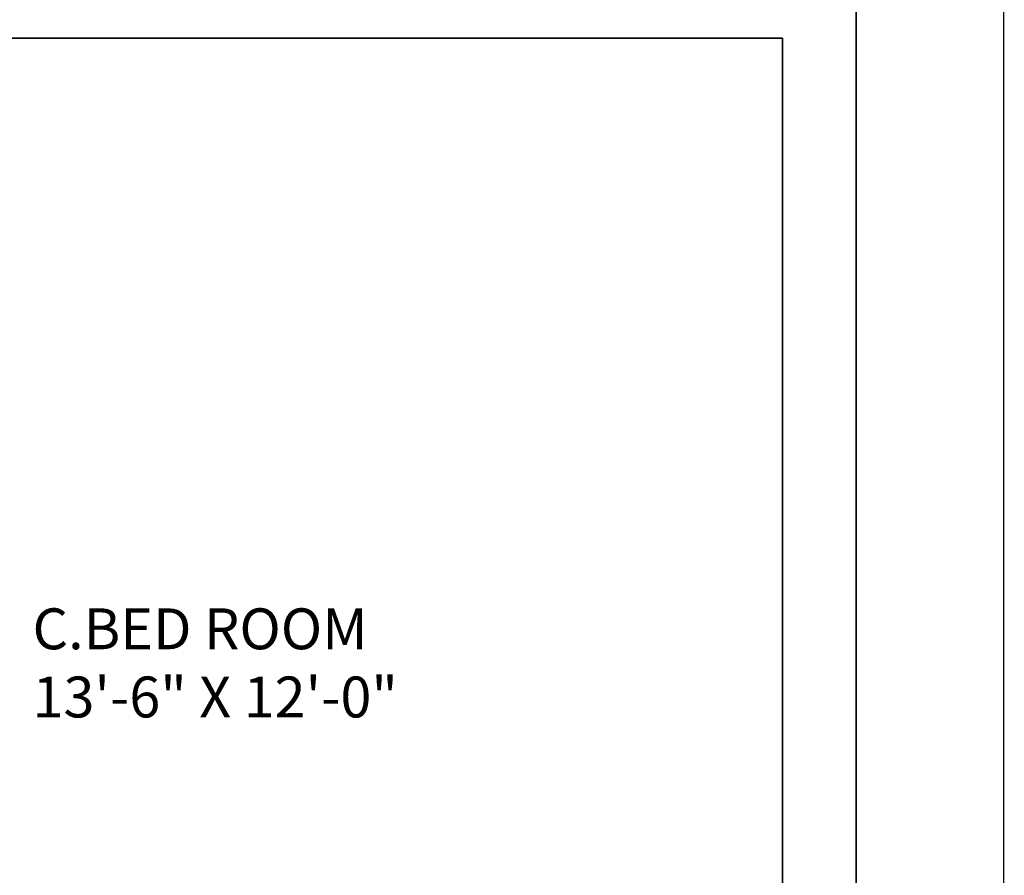
# Model space of a CAD drawing. Units: inches. Extents: x -638 to 186, y -762 to 59.
# Tile 20 of 31: x -92 to 29, y -308 to -203. Entities that reach past the tile are written whole.
import ezdxf

# ---------------------------------------------------------------- set-up
doc = ezdxf.new("R2010")
doc.units = ezdxf.units.IN
for name, color, linetype, lineweight in [('A-ANNO-DIMS', 2, 'Continuous', 18), ('A-AREA-IDEN', 1, 'Continuous', 18), ('C-PROP', 7, 'Continuous', 25), ('wall', 7, 'Continuous', 35)]:
    doc.layers.add(name, color=color, linetype=linetype, lineweight=lineweight)
doc.styles.get("Standard").update_dxf_attribs({"font": 'arial.ttf'})
doc.dimstyles.new('ISO-25', dxfattribs={"dimtxt": 4, "dimasz": 4, "dimexe": 1.25, "dimexo": 0.625, "dimtad": 0, "dimlunit": 4, "dimtxsty": 'Standard', "dimcen": 2.5, "dimclrt": 256, "dimadec": 0, "dimazin": 0, "dimtfac": 1, "dimtmove": 0, "dimatfit": 3, "dimfxl": 1, "dimfxlon": 1, "dimarcsym": 0})

# ---------------------------------------------------------------- blocks, each defined once
blk = doc.blocks.new('*D14')
at = {"layer": 'A-ANNO-DIMS', "color": 0, "lineweight": -2, "transparency": 16777216}
for p, q in [((45.41, -42.03), (47.66, -42.03)), ((46.41, -52.03), (46.41, -307.65)), ((46.41, -607.03), (46.41, -351.42)), ((45.41, -617.03), (47.66, -617.03))]:
    blk.add_line(p, q, dxfattribs=at)
at = {"layer": 'A-ANNO-DIMS', "color": 0, "lineweight": 30, "transparency": 16777216}
for points in [[(44.74, -52.03), (48.08, -52.03), (46.41, -42.03)], [(44.74, -607.03), (48.08, -607.03), (46.41, -617.03)]]:
    blk.add_solid(points, dxfattribs=at)
at = {"layer": 'Defpoints', "color": 0, "lineweight": 30, "transparency": 16777216}
for p in [(10.47, -42.03), (10.47, -617.03), (46.41, -617.03)]:
    blk.add_point(p, dxfattribs=at)
at = {"layer": 'A-ANNO-DIMS', "color": 0, "transparency": 16777216, "insert": (46.41, -329.53), "char_height": 10, "attachment_point": 5, "rotation": 90}
blk.add_mtext('47\'-11"', dxfattribs=at)
blk = doc.blocks.new('*D15')
at = {"layer": 'A-ANNO-DIMS', "color": 0, "lineweight": -2, "transparency": 16777216}
for p, q in [((69.33, -24.03), (71.58, -24.03)), ((70.33, -34.03), (70.33, -350.73)), ((70.33, -703.03), (70.33, -386.33)), ((69.33, -713.03), (71.58, -713.03))]:
    blk.add_line(p, q, dxfattribs=at)
at = {"layer": 'A-ANNO-DIMS', "color": 0, "lineweight": 30, "transparency": 16777216}
for points in [[(68.66, -34.03), (72, -34.03), (70.33, -24.03)], [(68.66, -703.03), (72, -703.03), (70.33, -713.03)]]:
    blk.add_solid(points, dxfattribs=at)
at = {"layer": 'Defpoints', "color": 0, "lineweight": 30, "transparency": 16777216}
for p in [(-24.67, -24.03), (-10.56, -713.03), (70.33, -713.03)]:
    blk.add_point(p, dxfattribs=at)
at = {"layer": 'A-ANNO-DIMS', "color": 0, "transparency": 16777216, "insert": (70.33, -368.53), "char_height": 10, "attachment_point": 5, "rotation": 90}
blk.add_mtext('57\'-5"', dxfattribs=at)
blk = doc.blocks.new('*D37')
at = {"layer": 'A-ANNO-DIMS', "color": 0, "lineweight": -2, "transparency": 16777216}
for p, q in [((182.66, -232.53), (184.91, -232.53)), ((183.66, -236.53), (183.66, -250.51)), ((183.66, -276.53), (183.66, -262.56)), ((182.66, -280.53), (184.91, -280.53))]:
    blk.add_line(p, q, dxfattribs=at)
at = {"layer": 'A-ANNO-DIMS', "color": 0, "lineweight": 30, "transparency": 16777216}
for points in [[(183, -236.53), (184.33, -236.53), (183.66, -232.53)], [(183, -276.53), (184.33, -276.53), (183.66, -280.53)]]:
    blk.add_solid(points, dxfattribs=at)
at = {"layer": 'Defpoints', "color": 0, "lineweight": 30, "transparency": 16777216}
for p in [(-404.53, -232.53), (-404.53, -280.53), (183.66, -280.53)]:
    blk.add_point(p, dxfattribs=at)
at = {"layer": 'A-ANNO-DIMS', "transparency": 16777216, "insert": (183.66, -256.53), "char_height": 4, "attachment_point": 5, "rotation": 90}
blk.add_mtext('4\'-0"', dxfattribs=at)
blk = doc.blocks.new('*D38')
at = {"layer": 'A-ANNO-DIMS', "color": 0, "lineweight": -2, "transparency": 16777216}
for p, q in [((182.66, -280.53), (184.91, -280.53)), ((183.66, -284.53), (183.66, -371.73)), ((183.66, -473.53), (183.66, -386.34)), ((182.66, -477.53), (184.91, -477.53))]:
    blk.add_line(p, q, dxfattribs=at)
at = {"layer": 'A-ANNO-DIMS', "color": 0, "lineweight": 30, "transparency": 16777216}
for points in [[(183, -284.53), (184.33, -284.53), (183.66, -280.53)], [(183, -473.53), (184.33, -473.53), (183.66, -477.53)]]:
    blk.add_solid(points, dxfattribs=at)
at = {"layer": 'Defpoints', "color": 0, "lineweight": 30, "transparency": 16777216}
for p in [(-404.53, -280.53), (-404.53, -477.53), (183.66, -477.53)]:
    blk.add_point(p, dxfattribs=at)
at = {"layer": 'A-ANNO-DIMS', "transparency": 16777216, "insert": (183.66, -379.03), "char_height": 4, "attachment_point": 5, "rotation": 90}
blk.add_mtext('16\'-5"', dxfattribs=at)

msp = doc.modelspace()

# ---------------------------------------------------------------- linework, layer by layer
at = {"layer": 'C-PROP'}
msp.add_line((28.474, -24.033), (28.474, -713.033), dxfattribs=at)
at = {"layer": 'wall'}
for p, q in [((10.474, -42.033), (10.474, -617.033)), ((-160.526, -205.533), (1.474, -205.533)), ((1.474, -205.533), (1.474, -349.533))]:
    msp.add_line(p, q, dxfattribs=at)

# ---------------------------------------------------------------- texts
at = {"layer": 'A-AREA-IDEN', "insert": (-90.258, -275.268), "char_height": 5, "attachment_point": 1}
msp.add_mtext_dynamic_manual_height_columns('{C.BED ROOM\\P13\'-6" X 12\'-0"}', width=101.0374, gutter_width=12.5, heights=[0], dxfattribs=at)

# ---------------------------------------------------------------- dimensions: what is measured, and where the dimension line sits
at = {"layer": 'A-ANNO-DIMS'}
for base, p1, p2, override, picture, middle in [((70.331, -713.033), (-24.669, -24.033), (-10.563, -713.033), {"dimtxt": 10, "dimasz": 10, "dimclrd": 0, "dimclre": 0, "dimclrt": 0}, '*D15', (70.331, -368.533)), ((46.411, -617.033), (10.474, -42.033), (10.474, -617.033), {"dimtxt": 10, "dimasz": 10, "dimclrd": 0, "dimclre": 0, "dimclrt": 0}, '*D14', (46.411, -329.533)), ((183.663, -280.533), (-404.526, -232.533), (-404.526, -280.533), {"dimdec": 1, "dimlfac": 1, "dimrnd": 0, "dimzin": 1, "dimdsep": 46, "dimlunit": 4, "dimfrac": 2}, '*D37', (183.663, -256.533)), ((183.663, -477.533), (-404.526, -280.533), (-404.526, -477.533), {"dimdec": 1, "dimlfac": 1, "dimrnd": 0, "dimzin": 1, "dimdsep": 46, "dimlunit": 4, "dimfrac": 2}, '*D38', (183.663, -379.033))]:
    dim = msp.add_linear_dim(base=base, p1=p1, p2=p2, angle=90, dimstyle='ISO-25', override=override, dxfattribs=at)
    dim.commit()
    dim.dimension.update_dxf_attribs({"geometry": picture, "text_midpoint": middle})

doc.saveas('drawing.dxf')
